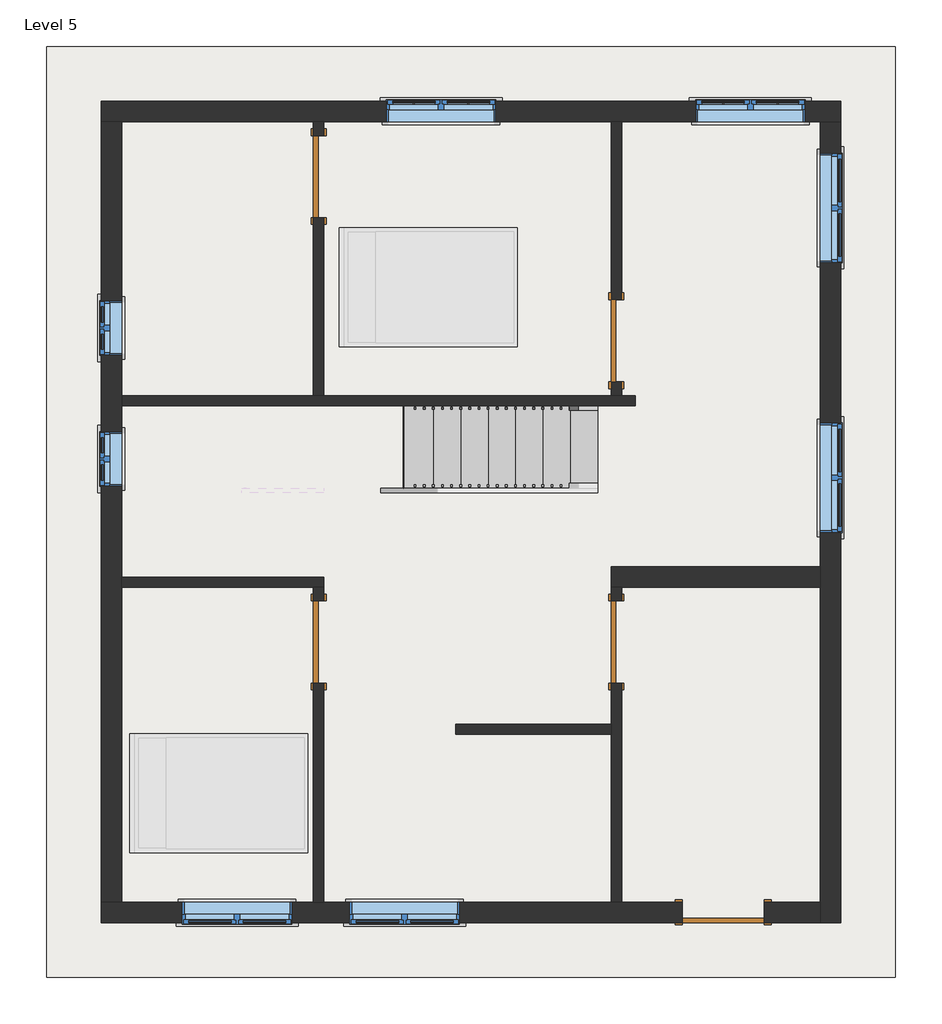
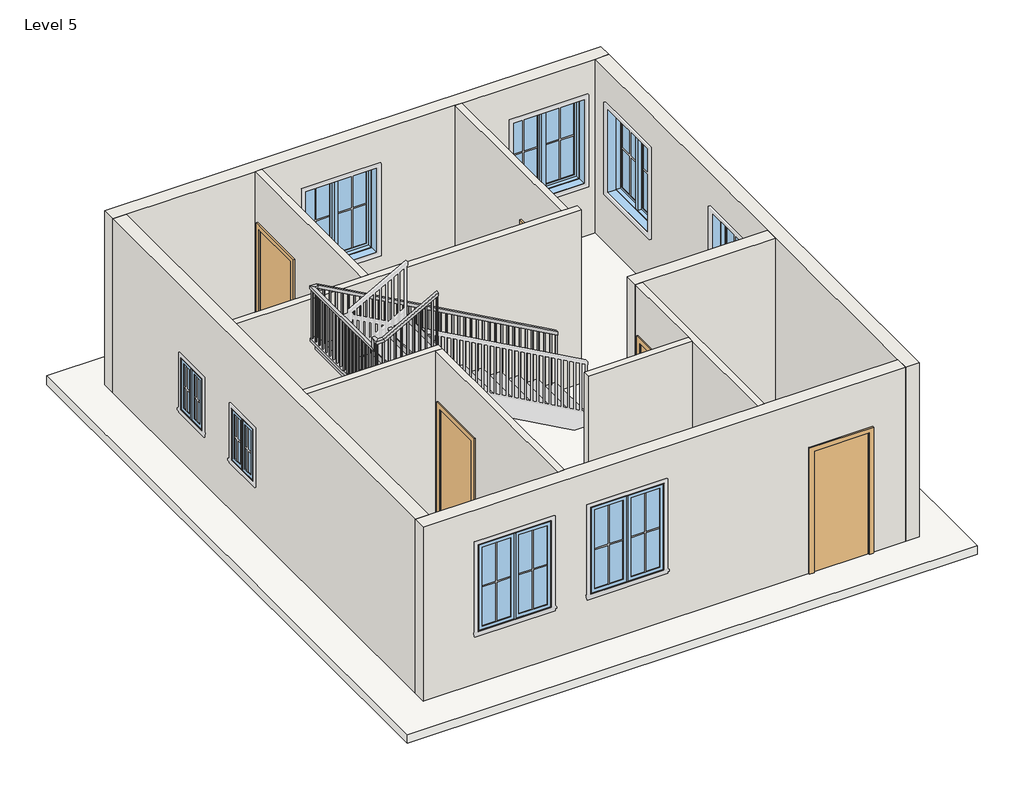
# One storey, part 1 of 2: 12 walls, 8 windows, 5 doors, 1 railing, 1 slab, 1 stair flight.
"""IFC4 building model written with IfcOpenShell, lengths in millimetres."""

from ifc_helpers import new_model, si_unit, frame, origin, place, context, project, spatial, polyline, outline, extrude, faceted_brep, transform, mapped, element, save
from components import door_e5f9f3c4, door_305aa2a5, door_0ca8825f, stair_flight_f65a8a44, window_c417fced, window_8377141f

model = new_model("IFC4")

# Units and contexts
model_context = context("Model", 3, world=origin())
ifc_project = project(units=[si_unit("LENGTHUNIT", "METRE", prefix="MILLI")], contexts=[model_context])

# Site, building, storey
site = spatial("IfcSite", under=ifc_project)
building = spatial("IfcBuilding", under=site)
storey = spatial("IfcBuildingStorey", under=building, Name="Level 5", Elevation=12192.0)

# Doors
placement = place(None, origin())
door_shape = door_e5f9f3c4(model_context)
element("IfcDoor", 1, ObjectType="Single-Flush : 36\" x 84\"", at=placement, inside=storey, context=model_context, shape_type="MappedRepresentation", body=[
    mapped(door_shape, transform((3689.35, 13938.7372886, 12192.0), x_axis=(0.0, 1.0, 0.0), y_axis=(-1.0, 0.0, 0.0), z_axis=(0.0, 0.0, 1.0))),
])
door_2_shape = door_305aa2a5(model_context)
element("IfcDoor", 2, ObjectType="Single-Flush : 36\" x 84\"", at=placement, inside=storey, context=model_context, shape_type="MappedRepresentation", body=[
    mapped(door_2_shape, transform((7004.05, 12109.9372886, 12192.0), x_axis=(0.0, -1.0, 0.0), y_axis=(1.0, 0.0, 0.0), z_axis=(0.0, 0.0, 1.0))),
])
element("IfcDoor", 3, ObjectType="Single-Flush : 36\" x 84\"", at=placement, inside=storey, context=model_context, shape_type="MappedRepresentation", body=[
    mapped(door_2_shape, transform((3689.3519847, 8757.1372886, 12192.0), x_axis=(0.0, -1.0, 0.0), y_axis=(1.0, 0.0, 0.0), z_axis=(0.0, 0.0, 1.0))),
])
element("IfcDoor", 4, ObjectType="Single-Flush : 36\" x 84\"", at=placement, inside=storey, context=model_context, shape_type="MappedRepresentation", body=[
    mapped(door_2_shape, transform((7004.05, 8757.1372886, 12192.0), x_axis=(0.0, -1.0, 0.0), y_axis=(1.0, 0.0, 0.0), z_axis=(0.0, 0.0, 1.0))),
])
door_3_shape = door_0ca8825f(model_context)
element("IfcDoor", 5, ObjectType="Single-Flush : 36\" x 84\"", at=placement, inside=storey, context=model_context, shape_type="MappedRepresentation", body=[
    mapped(door_3_shape, transform((8194.675, 5747.2372886, 12192.0), x_axis=(-1.0, 0.0, 0.0), y_axis=(0.0, -1.0, 0.0), z_axis=(0.0, 0.0, 1.0))),
])

# Railing
element("IfcRailing", 6, ObjectType="Handrail - Rectangular", at=placement, inside=storey, context=model_context, shape_type="SolidModel", body=[
    faceted_brep([(6794.5, 11335.2372886, 13275.7333333), (6794.5, 11335.2372886, 13217.620221), (6794.5, 11386.0372886, 13217.620221), (6794.5, 11386.0372886, 13275.7333333), (2832.1, 11335.2372886, 15477.0666667), (2818.9363978, 11335.2372886, 15426.2666667), (2818.9363978, 11386.0372886, 15426.2666667), (2832.1, 11386.0372886, 15477.0666667), (2768.6, 11335.2372886, 15477.0666667), (2768.6, 11335.2372886, 15426.2666667), (2717.8, 11386.0372886, 15426.2666667), (2717.8, 11386.0372886, 15477.0666667), (2768.6, 9608.0372886, 15477.0666667), (2768.6, 9557.2372886, 15426.2666667), (2717.8, 9557.2372886, 15426.2666667), (2717.8, 9608.0372886, 15477.0666667), (2768.6, 9608.0372886, 15653.4555402), (2768.6, 9557.2372886, 15602.6555402), (2717.8, 9557.2372886, 15602.6555402), (2717.8, 9608.0372886, 15653.4555402), (2768.6, 9531.8372886, 15653.4555402), (2768.6, 9531.8372886, 15602.6555402), (2717.8, 9481.0372886, 15602.6555402), (2717.8, 9481.0372886, 15653.4555402), (2844.8, 9531.8372886, 15653.4555402), (2857.9635773, 9531.8372886, 15602.6555402), (2857.9635773, 9481.0372886, 15602.6555402), (2844.8, 9481.0372886, 15653.4555402), (3746.5019847, 9531.8372886, 16154.4), (3746.5019847, 9481.0372886, 16154.4), (3746.5019847, 9481.0372886, 16096.2869174), (3746.5019847, 9531.8372886, 16096.2869174)], [[[0, 1, 2, 3]], [[1, 0, 4, 5]], [[2, 1, 5, 6]], [[3, 2, 6, 7]], [[0, 3, 7, 4]], [[5, 4, 8, 9]], [[6, 5, 9, 10]], [[7, 6, 10, 11]], [[4, 7, 11, 8]], [[9, 8, 12, 13]], [[10, 9, 13, 14]], [[11, 10, 14, 15]], [[8, 11, 15, 12]], [[13, 12, 16, 17]], [[14, 13, 17, 18]], [[15, 14, 18, 19]], [[12, 15, 19, 16]], [[17, 16, 20, 21]], [[18, 17, 21, 22]], [[19, 18, 22, 23]], [[16, 19, 23, 20]], [[21, 20, 24, 25]], [[22, 21, 25, 26]], [[23, 22, 26, 27]], [[20, 23, 27, 24]], [[28, 29, 30, 31]], [[25, 24, 28, 31]], [[26, 25, 31, 30]], [[27, 26, 30, 29]], [[24, 27, 29, 28]]]),
    extrude(outline(polyline([(16052.1894234, 3667.125), (16041.606113, 3648.075), (15070.6666667, 3648.075), (15070.6666667, 3667.125), (16052.1894234, 3667.125)])), frame((0.0, 9496.9122886, 0.0), z_axis=(0.0, 1.0, 0.0), x_axis=(0.0, 0.0, 1.0)), (0.0, 0.0, 1.0), 19.05),
    extrude(outline(polyline([(15995.7451014, 3565.525), (15985.1617911, 3546.475), (15070.6666667, 3546.475), (15070.6666667, 3565.525), (15995.7451014, 3565.525)])), frame((0.0, 9496.9122886, 0.0), z_axis=(0.0, 1.0, 0.0), x_axis=(0.0, 0.0, 1.0)), (0.0, 0.0, 1.0), 19.05),
    extrude(outline(polyline([(15939.3007795, 3463.925), (15928.7174691, 3444.875), (15070.6666667, 3444.875), (15070.6666667, 3463.925), (15939.3007795, 3463.925)])), frame((0.0, 9496.9122886, 0.0), z_axis=(0.0, 1.0, 0.0), x_axis=(0.0, 0.0, 1.0)), (0.0, 0.0, 1.0), 19.05),
    extrude(outline(polyline([(15882.85609, 3362.325), (15872.2727797, 3343.275), (14901.3333333, 3343.275), (14901.3333333, 3362.325), (15882.85609, 3362.325)])), frame((0.0, 9496.9122886, 0.0), z_axis=(0.0, 1.0, 0.0), x_axis=(0.0, 0.0, 1.0)), (0.0, 0.0, 1.0), 19.05),
    extrude(outline(polyline([(15826.4117681, 3260.725), (15815.8284577, 3241.675), (14901.3333333, 3241.675), (14901.3333333, 3260.725), (15826.4117681, 3260.725)])), frame((0.0, 9496.9122886, 0.0), z_axis=(0.0, 1.0, 0.0), x_axis=(0.0, 0.0, 1.0)), (0.0, 0.0, 1.0), 19.05),
    extrude(outline(polyline([(15769.9674462, 3159.125), (15759.3841358, 3140.075), (14901.3333333, 3140.075), (14901.3333333, 3159.125), (15769.9674462, 3159.125)])), frame((0.0, 9496.9122886, 0.0), z_axis=(0.0, 1.0, 0.0), x_axis=(0.0, 0.0, 1.0)), (0.0, 0.0, 1.0), 19.05),
    extrude(outline(polyline([(15713.5227567, 3057.525), (15702.9394463, 3038.475), (14732.0, 3038.475), (14732.0, 3057.525), (15713.5227567, 3057.525)])), frame((0.0, 9496.9122886, 0.0), z_axis=(0.0, 1.0, 0.0), x_axis=(0.0, 0.0, 1.0)), (0.0, 0.0, 1.0), 19.05),
    extrude(outline(polyline([(15657.0784348, 2955.925), (15646.4951244, 2936.875), (14732.0, 2936.875), (14732.0, 2955.925), (15657.0784348, 2955.925)])), frame((0.0, 9496.9122886, 0.0), z_axis=(0.0, 1.0, 0.0), x_axis=(0.0, 0.0, 1.0)), (0.0, 0.0, 1.0), 19.05),
    extrude(outline(polyline([(15600.6341128, 2854.325), (15590.0508025, 2835.275), (14732.0, 2835.275), (14732.0, 2854.325), (15600.6341128, 2854.325)])), frame((0.0, 9496.9122886, 0.0), z_axis=(0.0, 1.0, 0.0), x_axis=(0.0, 0.0, 1.0)), (0.0, 0.0, 1.0), 19.05),
    extrude(outline(polyline([(2733.675, 9541.3622886), (2752.725, 9541.3622886), (2752.725, 9522.3122886), (2733.675, 9522.3122886), (2733.675, 9541.3622886)])), frame((0.0, 0.0, 14562.6666667), z_axis=(0.0, 0.0, 1.0), x_axis=(1.0, 0.0, 0.0)), (0.0, 0.0, 1.0), 1039.9888736),
    extrude(outline(polyline([(2733.675, 9642.9622886), (2752.725, 9642.9622886), (2752.725, 9623.9122886), (2733.675, 9623.9122886), (2733.675, 9642.9622886)])), frame((0.0, 0.0, 14562.6666667), z_axis=(0.0, 0.0, 1.0), x_axis=(1.0, 0.0, 0.0)), (0.0, 0.0, 1.0), 863.6),
    extrude(outline(polyline([(2733.675, 9744.5622886), (2752.725, 9744.5622886), (2752.725, 9725.5122886), (2733.675, 9725.5122886), (2733.675, 9744.5622886)])), frame((0.0, 0.0, 14562.6666667), z_axis=(0.0, 0.0, 1.0), x_axis=(1.0, 0.0, 0.0)), (0.0, 0.0, 1.0), 863.6),
    extrude(outline(polyline([(2733.675, 9846.1622886), (2752.725, 9846.1622886), (2752.725, 9827.1122886), (2733.675, 9827.1122886), (2733.675, 9846.1622886)])), frame((0.0, 0.0, 14562.6666667), z_axis=(0.0, 0.0, 1.0), x_axis=(1.0, 0.0, 0.0)), (0.0, 0.0, 1.0), 863.6),
    extrude(outline(polyline([(2733.675, 9947.7622886), (2752.725, 9947.7622886), (2752.725, 9928.7122886), (2733.675, 9928.7122886), (2733.675, 9947.7622886)])), frame((0.0, 0.0, 14562.6666667), z_axis=(0.0, 0.0, 1.0), x_axis=(1.0, 0.0, 0.0)), (0.0, 0.0, 1.0), 863.6),
    extrude(outline(polyline([(2733.675, 10049.3622886), (2752.725, 10049.3622886), (2752.725, 10030.3122886), (2733.675, 10030.3122886), (2733.675, 10049.3622886)])), frame((0.0, 0.0, 14562.6666667), z_axis=(0.0, 0.0, 1.0), x_axis=(1.0, 0.0, 0.0)), (0.0, 0.0, 1.0), 863.6),
    extrude(outline(polyline([(2733.675, 10150.9622886), (2752.725, 10150.9622886), (2752.725, 10131.9122886), (2733.675, 10131.9122886), (2733.675, 10150.9622886)])), frame((0.0, 0.0, 14562.6666667), z_axis=(0.0, 0.0, 1.0), x_axis=(1.0, 0.0, 0.0)), (0.0, 0.0, 1.0), 863.6),
    extrude(outline(polyline([(2733.675, 10252.5622886), (2752.725, 10252.5622886), (2752.725, 10233.5122886), (2733.675, 10233.5122886), (2733.675, 10252.5622886)])), frame((0.0, 0.0, 14562.6666667), z_axis=(0.0, 0.0, 1.0), x_axis=(1.0, 0.0, 0.0)), (0.0, 0.0, 1.0), 863.6),
    extrude(outline(polyline([(2733.675, 10354.1622886), (2752.725, 10354.1622886), (2752.725, 10335.1122886), (2733.675, 10335.1122886), (2733.675, 10354.1622886)])), frame((0.0, 0.0, 14562.6666667), z_axis=(0.0, 0.0, 1.0), x_axis=(1.0, 0.0, 0.0)), (0.0, 0.0, 1.0), 863.6),
    extrude(outline(polyline([(2733.675, 10455.7622886), (2752.725, 10455.7622886), (2752.725, 10436.7122886), (2733.675, 10436.7122886), (2733.675, 10455.7622886)])), frame((0.0, 0.0, 14562.6666667), z_axis=(0.0, 0.0, 1.0), x_axis=(1.0, 0.0, 0.0)), (0.0, 0.0, 1.0), 863.6),
    extrude(outline(polyline([(2733.675, 10557.3622886), (2752.725, 10557.3622886), (2752.725, 10538.3122886), (2733.675, 10538.3122886), (2733.675, 10557.3622886)])), frame((0.0, 0.0, 14562.6666667), z_axis=(0.0, 0.0, 1.0), x_axis=(1.0, 0.0, 0.0)), (0.0, 0.0, 1.0), 863.6),
    extrude(outline(polyline([(2733.675, 10658.9622886), (2752.725, 10658.9622886), (2752.725, 10639.9122886), (2733.675, 10639.9122886), (2733.675, 10658.9622886)])), frame((0.0, 0.0, 14562.6666667), z_axis=(0.0, 0.0, 1.0), x_axis=(1.0, 0.0, 0.0)), (0.0, 0.0, 1.0), 863.6),
    extrude(outline(polyline([(2733.675, 10760.5622886), (2752.725, 10760.5622886), (2752.725, 10741.5122886), (2733.675, 10741.5122886), (2733.675, 10760.5622886)])), frame((0.0, 0.0, 14562.6666667), z_axis=(0.0, 0.0, 1.0), x_axis=(1.0, 0.0, 0.0)), (0.0, 0.0, 1.0), 863.6),
    extrude(outline(polyline([(2733.675, 10862.1622886), (2752.725, 10862.1622886), (2752.725, 10843.1122886), (2733.675, 10843.1122886), (2733.675, 10862.1622886)])), frame((0.0, 0.0, 14562.6666667), z_axis=(0.0, 0.0, 1.0), x_axis=(1.0, 0.0, 0.0)), (0.0, 0.0, 1.0), 863.6),
    extrude(outline(polyline([(2733.675, 10963.7622886), (2752.725, 10963.7622886), (2752.725, 10944.7122886), (2733.675, 10944.7122886), (2733.675, 10963.7622886)])), frame((0.0, 0.0, 14562.6666667), z_axis=(0.0, 0.0, 1.0), x_axis=(1.0, 0.0, 0.0)), (0.0, 0.0, 1.0), 863.6),
    extrude(outline(polyline([(2733.675, 11065.3622886), (2752.725, 11065.3622886), (2752.725, 11046.3122886), (2733.675, 11046.3122886), (2733.675, 11065.3622886)])), frame((0.0, 0.0, 14562.6666667), z_axis=(0.0, 0.0, 1.0), x_axis=(1.0, 0.0, 0.0)), (0.0, 0.0, 1.0), 863.6),
    extrude(outline(polyline([(2733.675, 11166.9622886), (2752.725, 11166.9622886), (2752.725, 11147.9122886), (2733.675, 11147.9122886), (2733.675, 11166.9622886)])), frame((0.0, 0.0, 14562.6666667), z_axis=(0.0, 0.0, 1.0), x_axis=(1.0, 0.0, 0.0)), (0.0, 0.0, 1.0), 863.6),
    extrude(outline(polyline([(2733.675, 11268.5622886), (2752.725, 11268.5622886), (2752.725, 11249.5122886), (2733.675, 11249.5122886), (2733.675, 11268.5622886)])), frame((0.0, 0.0, 14562.6666667), z_axis=(0.0, 0.0, 1.0), x_axis=(1.0, 0.0, 0.0)), (0.0, 0.0, 1.0), 863.6),
    extrude(outline(polyline([(15413.6618876, 2841.625), (15424.245221, 2822.575), (14562.6666667, 2822.575), (14562.6666667, 2841.625), (15413.6618876, 2841.625)])), frame((0.0, 11351.1122886, 0.0), z_axis=(0.0, 1.0, 0.0), x_axis=(0.0, 0.0, 1.0)), (0.0, 0.0, 1.0), 19.05),
    extrude(outline(polyline([(15357.2174432, 2943.225), (15367.8007765, 2924.175), (14393.3333333, 2924.175), (14393.3333333, 2943.225), (15357.2174432, 2943.225)])), frame((0.0, 11351.1122886, 0.0), z_axis=(0.0, 1.0, 0.0), x_axis=(0.0, 0.0, 1.0)), (0.0, 0.0, 1.0), 19.05),
    extrude(outline(polyline([(15300.7729988, 3044.825), (15311.3563321, 3025.775), (14393.3333333, 3025.775), (14393.3333333, 3044.825), (15300.7729988, 3044.825)])), frame((0.0, 11351.1122886, 0.0), z_axis=(0.0, 1.0, 0.0), x_axis=(0.0, 0.0, 1.0)), (0.0, 0.0, 1.0), 19.05),
    extrude(outline(polyline([(15244.3285543, 3146.425), (15254.9118876, 3127.375), (14393.3333333, 3127.375), (14393.3333333, 3146.425), (15244.3285543, 3146.425)])), frame((0.0, 11351.1122886, 0.0), z_axis=(0.0, 1.0, 0.0), x_axis=(0.0, 0.0, 1.0)), (0.0, 0.0, 1.0), 19.05),
    extrude(outline(polyline([(15187.8841099, 3248.025), (15198.4674432, 3228.975), (14224.0, 3228.975), (14224.0, 3248.025), (15187.8841099, 3248.025)])), frame((0.0, 11351.1122886, 0.0), z_axis=(0.0, 1.0, 0.0), x_axis=(0.0, 0.0, 1.0)), (0.0, 0.0, 1.0), 19.05),
    extrude(outline(polyline([(15131.4396654, 3349.625), (15142.0229988, 3330.575), (14224.0, 3330.575), (14224.0, 3349.625), (15131.4396654, 3349.625)])), frame((0.0, 11351.1122886, 0.0), z_axis=(0.0, 1.0, 0.0), x_axis=(0.0, 0.0, 1.0)), (0.0, 0.0, 1.0), 19.05),
    extrude(outline(polyline([(15074.995221, 3451.225), (15085.5785543, 3432.175), (14224.0, 3432.175), (14224.0, 3451.225), (15074.995221, 3451.225)])), frame((0.0, 11351.1122886, 0.0), z_axis=(0.0, 1.0, 0.0), x_axis=(0.0, 0.0, 1.0)), (0.0, 0.0, 1.0), 19.05),
    extrude(outline(polyline([(15018.5507765, 3552.825), (15029.1341099, 3533.775), (14054.6666667, 3533.775), (14054.6666667, 3552.825), (15018.5507765, 3552.825)])), frame((0.0, 11351.1122886, 0.0), z_axis=(0.0, 1.0, 0.0), x_axis=(0.0, 0.0, 1.0)), (0.0, 0.0, 1.0), 19.05),
    extrude(outline(polyline([(14962.1063321, 3654.425), (14972.6896654, 3635.375), (14054.6666667, 3635.375), (14054.6666667, 3654.425), (14962.1063321, 3654.425)])), frame((0.0, 11351.1122886, 0.0), z_axis=(0.0, 1.0, 0.0), x_axis=(0.0, 0.0, 1.0)), (0.0, 0.0, 1.0), 19.05),
    extrude(outline(polyline([(14905.6618876, 3756.025), (14916.245221, 3736.975), (14054.6666667, 3736.975), (14054.6666667, 3756.025), (14905.6618876, 3756.025)])), frame((0.0, 11351.1122886, 0.0), z_axis=(0.0, 1.0, 0.0), x_axis=(0.0, 0.0, 1.0)), (0.0, 0.0, 1.0), 19.05),
    extrude(outline(polyline([(14849.2174432, 3857.625), (14859.8007765, 3838.575), (13885.3333333, 3838.575), (13885.3333333, 3857.625), (14849.2174432, 3857.625)])), frame((0.0, 11351.1122886, 0.0), z_axis=(0.0, 1.0, 0.0), x_axis=(0.0, 0.0, 1.0)), (0.0, 0.0, 1.0), 19.05),
    extrude(outline(polyline([(14792.7729988, 3959.225), (14803.3563321, 3940.175), (13885.3333333, 3940.175), (13885.3333333, 3959.225), (14792.7729988, 3959.225)])), frame((0.0, 11351.1122886, 0.0), z_axis=(0.0, 1.0, 0.0), x_axis=(0.0, 0.0, 1.0)), (0.0, 0.0, 1.0), 19.05),
    extrude(outline(polyline([(14736.3285543, 4060.825), (14746.9118876, 4041.775), (13885.3333333, 4041.775), (13885.3333333, 4060.825), (14736.3285543, 4060.825)])), frame((0.0, 11351.1122886, 0.0), z_axis=(0.0, 1.0, 0.0), x_axis=(0.0, 0.0, 1.0)), (0.0, 0.0, 1.0), 19.05),
    extrude(outline(polyline([(14679.8841099, 4162.425), (14690.4674432, 4143.375), (13716.0, 4143.375), (13716.0, 4162.425), (14679.8841099, 4162.425)])), frame((0.0, 11351.1122886, 0.0), z_axis=(0.0, 1.0, 0.0), x_axis=(0.0, 0.0, 1.0)), (0.0, 0.0, 1.0), 19.05),
    extrude(outline(polyline([(14623.4396654, 4264.025), (14634.0229988, 4244.975), (13716.0, 4244.975), (13716.0, 4264.025), (14623.4396654, 4264.025)])), frame((0.0, 11351.1122886, 0.0), z_axis=(0.0, 1.0, 0.0), x_axis=(0.0, 0.0, 1.0)), (0.0, 0.0, 1.0), 19.05),
    extrude(outline(polyline([(14566.995221, 4365.625), (14577.5785543, 4346.575), (13716.0, 4346.575), (13716.0, 4365.625), (14566.995221, 4365.625)])), frame((0.0, 11351.1122886, 0.0), z_axis=(0.0, 1.0, 0.0), x_axis=(0.0, 0.0, 1.0)), (0.0, 0.0, 1.0), 19.05),
    extrude(outline(polyline([(14510.5507765, 4467.225), (14521.1341099, 4448.175), (13546.6666667, 4448.175), (13546.6666667, 4467.225), (14510.5507765, 4467.225)])), frame((0.0, 11351.1122886, 0.0), z_axis=(0.0, 1.0, 0.0), x_axis=(0.0, 0.0, 1.0)), (0.0, 0.0, 1.0), 19.05),
    extrude(outline(polyline([(14454.1063321, 4568.825), (14464.6896654, 4549.775), (13546.6666667, 4549.775), (13546.6666667, 4568.825), (14454.1063321, 4568.825)])), frame((0.0, 11351.1122886, 0.0), z_axis=(0.0, 1.0, 0.0), x_axis=(0.0, 0.0, 1.0)), (0.0, 0.0, 1.0), 19.05),
    extrude(outline(polyline([(14397.6618876, 4670.425), (14408.245221, 4651.375), (13546.6666667, 4651.375), (13546.6666667, 4670.425), (14397.6618876, 4670.425)])), frame((0.0, 11351.1122886, 0.0), z_axis=(0.0, 1.0, 0.0), x_axis=(0.0, 0.0, 1.0)), (0.0, 0.0, 1.0), 19.05),
    extrude(outline(polyline([(14341.2174432, 4772.025), (14351.8007765, 4752.975), (13377.3333333, 4752.975), (13377.3333333, 4772.025), (14341.2174432, 4772.025)])), frame((0.0, 11351.1122886, 0.0), z_axis=(0.0, 1.0, 0.0), x_axis=(0.0, 0.0, 1.0)), (0.0, 0.0, 1.0), 19.05),
    extrude(outline(polyline([(14284.7729988, 4873.625), (14295.3563321, 4854.575), (13377.3333333, 4854.575), (13377.3333333, 4873.625), (14284.7729988, 4873.625)])), frame((0.0, 11351.1122886, 0.0), z_axis=(0.0, 1.0, 0.0), x_axis=(0.0, 0.0, 1.0)), (0.0, 0.0, 1.0), 19.05),
    extrude(outline(polyline([(14228.3285543, 4975.225), (14238.9118876, 4956.175), (13377.3333333, 4956.175), (13377.3333333, 4975.225), (14228.3285543, 4975.225)])), frame((0.0, 11351.1122886, 0.0), z_axis=(0.0, 1.0, 0.0), x_axis=(0.0, 0.0, 1.0)), (0.0, 0.0, 1.0), 19.05),
    extrude(outline(polyline([(14171.8841099, 5076.825), (14182.4674432, 5057.775), (13208.0, 5057.775), (13208.0, 5076.825), (14171.8841099, 5076.825)])), frame((0.0, 11351.1122886, 0.0), z_axis=(0.0, 1.0, 0.0), x_axis=(0.0, 0.0, 1.0)), (0.0, 0.0, 1.0), 19.05),
    extrude(outline(polyline([(14115.4396654, 5178.425), (14126.0229988, 5159.375), (13208.0, 5159.375), (13208.0, 5178.425), (14115.4396654, 5178.425)])), frame((0.0, 11351.1122886, 0.0), z_axis=(0.0, 1.0, 0.0), x_axis=(0.0, 0.0, 1.0)), (0.0, 0.0, 1.0), 19.05),
    extrude(outline(polyline([(14058.995221, 5280.025), (14069.5785543, 5260.975), (13208.0, 5260.975), (13208.0, 5280.025), (14058.995221, 5280.025)])), frame((0.0, 11351.1122886, 0.0), z_axis=(0.0, 1.0, 0.0), x_axis=(0.0, 0.0, 1.0)), (0.0, 0.0, 1.0), 19.05),
    extrude(outline(polyline([(14002.5507765, 5381.625), (14013.1341099, 5362.575), (13038.6666667, 5362.575), (13038.6666667, 5381.625), (14002.5507765, 5381.625)])), frame((0.0, 11351.1122886, 0.0), z_axis=(0.0, 1.0, 0.0), x_axis=(0.0, 0.0, 1.0)), (0.0, 0.0, 1.0), 19.05),
    extrude(outline(polyline([(13946.1063321, 5483.225), (13956.6896654, 5464.175), (13038.6666667, 5464.175), (13038.6666667, 5483.225), (13946.1063321, 5483.225)])), frame((0.0, 11351.1122886, 0.0), z_axis=(0.0, 1.0, 0.0), x_axis=(0.0, 0.0, 1.0)), (0.0, 0.0, 1.0), 19.05),
    extrude(outline(polyline([(13889.6618876, 5584.825), (13900.245221, 5565.775), (13038.6666667, 5565.775), (13038.6666667, 5584.825), (13889.6618876, 5584.825)])), frame((0.0, 11351.1122886, 0.0), z_axis=(0.0, 1.0, 0.0), x_axis=(0.0, 0.0, 1.0)), (0.0, 0.0, 1.0), 19.05),
    extrude(outline(polyline([(13833.2174432, 5686.425), (13843.8007765, 5667.375), (12869.3333333, 5667.375), (12869.3333333, 5686.425), (13833.2174432, 5686.425)])), frame((0.0, 11351.1122886, 0.0), z_axis=(0.0, 1.0, 0.0), x_axis=(0.0, 0.0, 1.0)), (0.0, 0.0, 1.0), 19.05),
    extrude(outline(polyline([(13776.7729988, 5788.025), (13787.3563321, 5768.975), (12869.3333333, 5768.975), (12869.3333333, 5788.025), (13776.7729988, 5788.025)])), frame((0.0, 11351.1122886, 0.0), z_axis=(0.0, 1.0, 0.0), x_axis=(0.0, 0.0, 1.0)), (0.0, 0.0, 1.0), 19.05),
    extrude(outline(polyline([(13720.3285543, 5889.625), (13730.9118876, 5870.575), (12869.3333333, 5870.575), (12869.3333333, 5889.625), (13720.3285543, 5889.625)])), frame((0.0, 11351.1122886, 0.0), z_axis=(0.0, 1.0, 0.0), x_axis=(0.0, 0.0, 1.0)), (0.0, 0.0, 1.0), 19.05),
    extrude(outline(polyline([(13663.8841099, 5991.225), (13674.4674432, 5972.175), (12700.0, 5972.175), (12700.0, 5991.225), (13663.8841099, 5991.225)])), frame((0.0, 11351.1122886, 0.0), z_axis=(0.0, 1.0, 0.0), x_axis=(0.0, 0.0, 1.0)), (0.0, 0.0, 1.0), 19.05),
    extrude(outline(polyline([(13607.4396654, 6092.825), (13618.0229988, 6073.775), (12700.0, 6073.775), (12700.0, 6092.825), (13607.4396654, 6092.825)])), frame((0.0, 11351.1122886, 0.0), z_axis=(0.0, 1.0, 0.0), x_axis=(0.0, 0.0, 1.0)), (0.0, 0.0, 1.0), 19.05),
    extrude(outline(polyline([(13550.995221, 6194.425), (13561.5785543, 6175.375), (12700.0, 6175.375), (12700.0, 6194.425), (13550.995221, 6194.425)])), frame((0.0, 11351.1122886, 0.0), z_axis=(0.0, 1.0, 0.0), x_axis=(0.0, 0.0, 1.0)), (0.0, 0.0, 1.0), 19.05),
    extrude(outline(polyline([(13494.5507765, 6296.025), (13505.1341099, 6276.975), (12530.6666667, 6276.975), (12530.6666667, 6296.025), (13494.5507765, 6296.025)])), frame((0.0, 11351.1122886, 0.0), z_axis=(0.0, 1.0, 0.0), x_axis=(0.0, 0.0, 1.0)), (0.0, 0.0, 1.0), 19.05),
    extrude(outline(polyline([(13438.1063321, 6397.625), (13448.6896654, 6378.575), (12530.6666667, 6378.575), (12530.6666667, 6397.625), (13438.1063321, 6397.625)])), frame((0.0, 11351.1122886, 0.0), z_axis=(0.0, 1.0, 0.0), x_axis=(0.0, 0.0, 1.0)), (0.0, 0.0, 1.0), 19.05),
    extrude(outline(polyline([(13381.6618876, 6499.225), (13392.245221, 6480.175), (12530.6666667, 6480.175), (12530.6666667, 6499.225), (13381.6618876, 6499.225)])), frame((0.0, 11351.1122886, 0.0), z_axis=(0.0, 1.0, 0.0), x_axis=(0.0, 0.0, 1.0)), (0.0, 0.0, 1.0), 19.05),
    extrude(outline(polyline([(13325.2174432, 6600.825), (13335.8007765, 6581.775), (12361.3333333, 6581.775), (12361.3333333, 6600.825), (13325.2174432, 6600.825)])), frame((0.0, 11351.1122886, 0.0), z_axis=(0.0, 1.0, 0.0), x_axis=(0.0, 0.0, 1.0)), (0.0, 0.0, 1.0), 19.05),
    extrude(outline(polyline([(13268.7729988, 6702.425), (13279.3563321, 6683.375), (12361.3333333, 6683.375), (12361.3333333, 6702.425), (13268.7729988, 6702.425)])), frame((0.0, 11351.1122886, 0.0), z_axis=(0.0, 1.0, 0.0), x_axis=(0.0, 0.0, 1.0)), (0.0, 0.0, 1.0), 19.05),
    extrude(outline(polyline([(2733.675, 9515.9622886), (2752.725, 9515.9622886), (2752.725, 9496.9122886), (2733.675, 9496.9122886), (2733.675, 9515.9622886)])), frame((0.0, 0.0, 14562.6666667), z_axis=(0.0, 0.0, 1.0), x_axis=(1.0, 0.0, 0.0)), (0.0, 0.0, 1.0), 1039.9888736),
    extrude(outline(polyline([(2752.725, 11370.1622886), (2752.725, 11351.1122886), (2733.675, 11351.1122886), (2733.675, 11370.1622886), (2752.725, 11370.1622886)])), frame((0.0, 0.0, 14562.6666667), z_axis=(0.0, 0.0, 1.0), x_axis=(1.0, 0.0, 0.0)), (0.0, 0.0, 1.0), 863.6),
    extrude(outline(polyline([(16096.2869174, 3746.5019847), (16085.703607, 3727.4519847), (15070.6666667, 3727.4519847), (15070.6666667, 3746.5019847), (16096.2869174, 3746.5019847)])), frame((0.0, 9496.9122886, 0.0), z_axis=(0.0, 1.0, 0.0), x_axis=(0.0, 0.0, 1.0)), (0.0, 0.0, 1.0), 19.05),
    extrude(outline(polyline([(13217.620221, 6794.5), (13228.2035543, 6775.45), (12361.3333333, 6775.45), (12361.3333333, 6794.5), (13217.620221, 6794.5)])), frame((0.0, 11351.1122886, 0.0), z_axis=(0.0, 1.0, 0.0), x_axis=(0.0, 0.0, 1.0)), (0.0, 0.0, 1.0), 19.05),
])

# Slab
element("IfcSlab", 7, ObjectType="Generic - 12\"", at=placement, inside=storey, context=model_context, shape_type="SweptSolid", body=[
    extrude(outline(polyline([(10109.2, 15386.5372886), (10109.2, 5023.3372886), (660.4, 5023.3372886), (660.4, 15386.5372886), (10109.2, 15386.5372886)])), frame((0.0, 0.0, 12039.6), z_axis=(0.0, 0.0, 1.0), x_axis=(1.0, 0.0, 0.0)), (0.0, 0.0, 1.0), 152.4),
])

# Stair flight
stair_flight_shape = stair_flight_f65a8a44(model_context)
element("IfcStairFlight", 8, ObjectType="2\" Tread 1\" Nosing 1/4\" Riser", at=placement, inside=storey, context=model_context, shape_type="MappedRepresentation", body=[
    mapped(stair_flight_shape, transform((0.0, 0.0, 0.0), x_axis=(1.0, 0.0, 0.0), y_axis=(0.0, 1.0, 0.0), z_axis=(0.0, 0.0, 1.0))),
])

# Walls
element("IfcWall", 9, ObjectType="Generic - 5\"", at=placement, inside=storey, context=model_context, shape_type="SweptSolid", body=[
    extrude(outline(polyline([(14548.3372886, 12192.0), (14395.9372886, 12192.0), (14395.9372886, 14325.6), (13481.5372886, 14325.6), (13481.5372886, 12192.0), (11500.3372886, 12192.0), (11500.3372886, 15240.0), (14548.3372886, 15240.0), (14548.3372886, 12192.0)])), frame((3632.2, 0.0, 0.0), z_axis=(1.0, 0.0, 0.0), x_axis=(0.0, 1.0, 0.0)), (0.0, 0.0, 1.0), 114.3),
])
element("IfcWall", 10, ObjectType="Generic - 5\"", at=placement, inside=storey, context=model_context, shape_type="SweptSolid", body=[
    extrude(outline(polyline([(11652.7372886, 14325.6), (11652.7372886, 12192.0), (11500.3372886, 12192.0), (11500.3372886, 15240.0), (14548.3372886, 15240.0), (14548.3372886, 12192.0), (12567.1372886, 12192.0), (12567.1372886, 14325.6), (11652.7372886, 14325.6)])), frame((6946.9, 0.0, 0.0), z_axis=(1.0, 0.0, 0.0), x_axis=(0.0, 1.0, 0.0)), (0.0, 0.0, 1.0), 114.3),
])
element("IfcWall", 11, ObjectType="Generic - 5\"", at=placement, inside=storey, context=model_context, shape_type="Brep", body=[
    faceted_brep([(1498.6, 11386.0372886, 12192.0), (7213.6, 11386.0372886, 12192.0), (7213.6, 11386.0372886, 15240.0), (1498.6, 11386.0372886, 15240.0), (1498.6, 11500.3372886, 12192.0), (1498.6, 11500.3372886, 15240.0), (3632.2, 11500.3372886, 15240.0), (3746.5, 11500.3372886, 15240.0), (6946.9, 11500.3372886, 15240.0), (7061.2, 11500.3372886, 15240.0), (7213.6, 11500.3372886, 15240.0), (7213.6, 11500.3372886, 12192.0), (7061.2, 11500.3372886, 12192.0), (6946.9, 11500.3372886, 12192.0), (3746.5, 11500.3372886, 12192.0), (3632.2, 11500.3372886, 12192.0)], [[[0, 1, 2, 3]], [[4, 5, 6, 7, 8, 9, 10, 11, 12, 13, 14, 15]], [[1, 0, 4, 15, 14, 13, 12, 11]], [[2, 1, 11, 10]], [[3, 2, 10, 9, 8, 7, 6, 5]], [[0, 3, 5, 4]]]),
])
element("IfcWall", 12, ObjectType="Generic - 5\"", at=placement, inside=storey, context=model_context, shape_type="Brep", body=[
    faceted_brep([(1498.6, 9366.7372886, 12192.0), (3632.2019847, 9366.7372886, 12192.0), (3746.5019847, 9366.7372886, 12192.0), (3746.5019847, 9366.7372886, 15240.0), (3632.2019847, 9366.7372886, 15240.0), (1498.6, 9366.7372886, 15240.0), (1498.6, 9481.0372886, 12192.0), (1498.6, 9481.0372886, 15240.0), (3746.5019847, 9481.0372886, 15240.0), (3746.5019847, 9481.0372886, 12192.0)], [[[0, 1, 2, 3, 4, 5]], [[6, 7, 8, 9]], [[2, 1, 0, 6, 9]], [[5, 4, 3, 8, 7]], [[0, 5, 7, 6]], [[3, 2, 9, 8]]]),
])
element("IfcWall", 13, ObjectType="Generic - 5\"", at=placement, inside=storey, context=model_context, shape_type="SweptSolid", body=[
    extrude(outline(polyline([(8299.9372886, 14325.6), (8299.9372886, 12192.0), (5861.5372886, 12192.0), (5861.5372886, 15240.0), (9366.7372886, 15240.0), (9366.7372886, 12192.0), (9214.3372886, 12192.0), (9214.3372886, 14325.6), (8299.9372886, 14325.6)])), frame((3632.2019847, 0.0, 0.0), z_axis=(1.0, 0.0, 0.0), x_axis=(0.0, 1.0, 0.0)), (0.0, 0.0, 1.0), 114.3),
])
element("IfcWall", 14, ObjectType="Generic - 5\"", at=placement, inside=storey, context=model_context, shape_type="Brep", body=[
    faceted_brep([(7061.2, 5861.5372886, 12192.0), (7061.2, 8299.9372886, 12192.0), (7061.2, 8299.9372886, 14325.6), (7061.2, 9214.3372886, 14325.6), (7061.2, 9214.3372886, 12192.0), (7061.2, 9366.7372886, 12192.0), (7061.2, 9366.7372886, 15240.0), (7061.2, 5861.5372886, 15240.0), (6946.9, 8299.9372886, 14325.6), (6946.9, 8299.9372886, 12192.0), (6946.9, 7842.7372886, 12192.0), (6946.9, 7728.4372886, 12192.0), (6946.9, 5861.5372886, 12192.0), (6946.9, 5861.5372886, 15240.0), (6946.9, 7728.4372886, 15240.0), (6946.9, 7842.7372886, 15240.0), (6946.9, 9366.7372886, 15240.0), (6946.9, 9366.7372886, 12192.0), (6946.9, 9214.3372886, 12192.0), (6946.9, 9214.3372886, 14325.6)], [[[0, 1, 2, 3, 4, 5, 6, 7]], [[8, 9, 10, 11, 12, 13, 14, 15, 16, 17, 18, 19]], [[18, 17, 5, 4]], [[12, 11, 10, 9, 1, 0]], [[7, 6, 16, 15, 14, 13]], [[0, 7, 13, 12]], [[6, 5, 17, 16]], [[2, 1, 9, 8]], [[3, 2, 8, 19]], [[4, 3, 19, 18]]]),
])
element("IfcWall", 15, ObjectType="Generic - 5\"", at=placement, inside=storey, context=model_context, shape_type="SweptSolid", body=[
    extrude(outline(polyline([(5215.2207778, 7842.7372886), (6946.9, 7842.7372886), (6946.9, 7728.4372886), (5215.2207778, 7728.4372886), (5215.2207778, 7842.7372886)])), frame((0.0, 0.0, 12192.0), z_axis=(0.0, 0.0, 1.0), x_axis=(1.0, 0.0, 0.0)), (0.0, 0.0, 1.0), 3048.0),
])
element("IfcWall", 16, ObjectType="Generic - 8\"", at=placement, inside=storey, context=model_context, shape_type="Brep", body=[
    faceted_brep([(1270.0, 14548.3372886, 12192.0), (1498.6, 14548.3372886, 12192.0), (3632.2, 14548.3372886, 12192.0), (3746.5, 14548.3372886, 12192.0), (6946.9, 14548.3372886, 12192.0), (7061.2, 14548.3372886, 12192.0), (9271.0, 14548.3372886, 12192.0), (9499.6, 14548.3372886, 12192.0), (9499.6, 14548.3372886, 15240.0), (9271.0, 14548.3372886, 15240.0), (7061.2, 14548.3372886, 15240.0), (6946.9, 14548.3372886, 15240.0), (3746.5, 14548.3372886, 15240.0), (3632.2, 14548.3372886, 15240.0), (1498.6, 14548.3372886, 15240.0), (1270.0, 14548.3372886, 15240.0), (9105.9, 14548.3372886, 14630.4), (9105.9, 14548.3372886, 13106.4), (7886.7, 14548.3372886, 13106.4), (7886.7, 14548.3372886, 14630.4), (5662.6125, 14548.3372886, 14630.4), (5662.6125, 14548.3372886, 13106.4), (4443.4125, 14548.3372886, 13106.4), (4443.4125, 14548.3372886, 14630.4), (1270.0, 14776.9372886, 12192.0), (1270.0, 14776.9372886, 15240.0), (9499.6, 14776.9372886, 15240.0), (9499.6, 14776.9372886, 12192.0), (9105.9, 14776.9372886, 14630.4), (7886.7, 14776.9372886, 14630.4), (7886.7, 14776.9372886, 13106.4), (9105.9, 14776.9372886, 13106.4), (5662.6125, 14776.9372886, 14630.4), (4443.4125, 14776.9372886, 14630.4), (4443.4125, 14776.9372886, 13106.4), (5662.6125, 14776.9372886, 13106.4)], [[[0, 1, 2, 3, 4, 5, 6, 7, 8, 9, 10, 11, 12, 13, 14, 15], [16, 17, 18, 19], [20, 21, 22, 23]], [[24, 25, 26, 27], [28, 29, 30, 31], [32, 33, 34, 35]], [[7, 6, 5, 4, 3, 2, 1, 0, 24, 27]], [[8, 7, 27, 26]], [[0, 15, 25, 24]], [[17, 16, 28, 31]], [[18, 17, 31, 30]], [[19, 18, 30, 29]], [[16, 19, 29, 28]], [[21, 20, 32, 35]], [[22, 21, 35, 34]], [[23, 22, 34, 33]], [[20, 23, 33, 32]], [[15, 14, 13, 12, 11, 10, 9, 8, 26, 25]]]),
])
element("IfcWall", 17, ObjectType="Generic - 8\"", at=placement, inside=storey, context=model_context, shape_type="Brep", body=[
    faceted_brep([(9271.0, 14548.3372886, 12192.0), (9271.0, 9595.3372886, 12192.0), (9271.0, 9366.7372886, 12192.0), (9271.0, 5861.5372886, 12192.0), (9271.0, 5632.9372886, 12192.0), (9271.0, 5632.9372886, 15240.0), (9271.0, 5861.5372886, 15240.0), (9271.0, 9366.7372886, 15240.0), (9271.0, 9595.3372886, 15240.0), (9271.0, 14548.3372886, 15240.0), (9271.0, 12979.8872886, 14630.4), (9271.0, 12979.8872886, 13106.4), (9271.0, 14199.0872886, 13106.4), (9271.0, 14199.0872886, 14630.4), (9271.0, 9976.3372886, 14630.4), (9271.0, 9976.3372886, 13106.4), (9271.0, 11195.5372886, 13106.4), (9271.0, 11195.5372886, 14630.4), (9499.6, 14548.3372886, 12192.0), (9499.6, 14548.3372886, 15240.0), (9499.6, 5632.9372886, 15240.0), (9499.6, 5632.9372886, 12192.0), (9499.6, 12979.8872886, 14630.4), (9499.6, 14199.0872886, 14630.4), (9499.6, 14199.0872886, 13106.4), (9499.6, 12979.8872886, 13106.4), (9499.6, 9976.3372886, 14630.4), (9499.6, 11195.5372886, 14630.4), (9499.6, 11195.5372886, 13106.4), (9499.6, 9976.3372886, 13106.4)], [[[0, 1, 2, 3, 4, 5, 6, 7, 8, 9], [10, 11, 12, 13], [14, 15, 16, 17]], [[18, 19, 20, 21], [22, 23, 24, 25], [26, 27, 28, 29]], [[4, 3, 2, 1, 0, 18, 21]], [[0, 9, 19, 18]], [[5, 4, 21, 20]], [[11, 10, 22, 25]], [[12, 11, 25, 24]], [[13, 12, 24, 23]], [[10, 13, 23, 22]], [[15, 14, 26, 29]], [[16, 15, 29, 28]], [[17, 16, 28, 27]], [[14, 17, 27, 26]], [[9, 8, 7, 6, 5, 20, 19]]]),
])
element("IfcWall", 18, ObjectType="Generic - 8\"", at=placement, inside=storey, context=model_context, shape_type="Brep", body=[
    faceted_brep([(7737.475, 5861.5372886, 14325.6), (7737.475, 5861.5372886, 12192.0), (7061.2, 5861.5372886, 12192.0), (6946.9, 5861.5372886, 12192.0), (3746.5019847, 5861.5372886, 12192.0), (3632.2019847, 5861.5372886, 12192.0), (1498.6, 5861.5372886, 12192.0), (1270.0, 5861.5372886, 12192.0), (1270.0, 5861.5372886, 15240.0), (1498.6, 5861.5372886, 15240.0), (3632.2019847, 5861.5372886, 15240.0), (3746.5019847, 5861.5372886, 15240.0), (6946.9, 5861.5372886, 15240.0), (7061.2, 5861.5372886, 15240.0), (9271.0, 5861.5372886, 15240.0), (9271.0, 5861.5372886, 12192.0), (8651.875, 5861.5372886, 12192.0), (8651.875, 5861.5372886, 14325.6), (4037.8082347, 5861.5372886, 14630.4), (4037.8082347, 5861.5372886, 13106.4), (5257.0082347, 5861.5372886, 13106.4), (5257.0082347, 5861.5372886, 14630.4), (2173.2894847, 5861.5372886, 14630.4), (2173.2894847, 5861.5372886, 13106.4), (3392.4894847, 5861.5372886, 13106.4), (3392.4894847, 5861.5372886, 14630.4), (1270.0, 5632.9372886, 12192.0), (7737.475, 5632.9372886, 12192.0), (7737.475, 5632.9372886, 14325.6), (8651.875, 5632.9372886, 14325.6), (8651.875, 5632.9372886, 12192.0), (9271.0, 5632.9372886, 12192.0), (9271.0, 5632.9372886, 15240.0), (1270.0, 5632.9372886, 15240.0), (4037.8082347, 5632.9372886, 14630.4), (5257.0082347, 5632.9372886, 14630.4), (5257.0082347, 5632.9372886, 13106.4), (4037.8082347, 5632.9372886, 13106.4), (2173.2894847, 5632.9372886, 14630.4), (3392.4894847, 5632.9372886, 14630.4), (3392.4894847, 5632.9372886, 13106.4), (2173.2894847, 5632.9372886, 13106.4)], [[[0, 1, 2, 3, 4, 5, 6, 7, 8, 9, 10, 11, 12, 13, 14, 15, 16, 17], [18, 19, 20, 21], [22, 23, 24, 25]], [[26, 27, 28, 29, 30, 31, 32, 33], [34, 35, 36, 37], [38, 39, 40, 41]], [[16, 15, 31, 30]], [[7, 6, 5, 4, 3, 2, 1, 27, 26]], [[15, 14, 32, 31]], [[8, 7, 26, 33]], [[19, 18, 34, 37]], [[20, 19, 37, 36]], [[21, 20, 36, 35]], [[18, 21, 35, 34]], [[23, 22, 38, 41]], [[24, 23, 41, 40]], [[25, 24, 40, 39]], [[22, 25, 39, 38]], [[14, 13, 12, 11, 10, 9, 8, 33, 32]], [[28, 27, 1, 0]], [[29, 28, 0, 17]], [[30, 29, 17, 16]]]),
])
element("IfcWall", 19, ObjectType="Generic - 8\"", at=placement, inside=storey, context=model_context, shape_type="Brep", body=[
    faceted_brep([(1498.6, 5861.5372886, 12192.0), (1498.6, 9366.7372886, 12192.0), (1498.6, 9481.0372886, 12192.0), (1498.6, 11386.0372886, 12192.0), (1498.6, 11500.3372886, 12192.0), (1498.6, 14548.3372886, 12192.0), (1498.6, 14548.3372886, 15240.0), (1498.6, 11500.3372886, 15240.0), (1498.6, 11386.0372886, 15240.0), (1498.6, 9481.0372886, 15240.0), (1498.6, 9366.7372886, 15240.0), (1498.6, 5861.5372886, 15240.0), (1498.6, 12557.6122886, 14020.8), (1498.6, 12557.6122886, 13106.4), (1498.6, 11948.0122886, 13106.4), (1498.6, 11948.0122886, 14020.8), (1498.6, 11100.2872886, 14020.8), (1498.6, 11100.2872886, 13106.4), (1498.6, 10490.6872886, 13106.4), (1498.6, 10490.6872886, 14020.8), (1270.0, 5861.5372886, 12192.0), (1270.0, 5861.5372886, 15240.0), (1270.0, 14548.3372886, 15240.0), (1270.0, 14548.3372886, 12192.0), (1270.0, 12557.6122886, 14020.8), (1270.0, 11948.0122886, 14020.8), (1270.0, 11948.0122886, 13106.4), (1270.0, 12557.6122886, 13106.4), (1270.0, 11100.2872886, 14020.8), (1270.0, 10490.6872886, 14020.8), (1270.0, 10490.6872886, 13106.4), (1270.0, 11100.2872886, 13106.4)], [[[0, 1, 2, 3, 4, 5, 6, 7, 8, 9, 10, 11], [12, 13, 14, 15], [16, 17, 18, 19]], [[20, 21, 22, 23], [24, 25, 26, 27], [28, 29, 30, 31]], [[5, 4, 3, 2, 1, 0, 20, 23]], [[6, 5, 23, 22]], [[0, 11, 21, 20]], [[13, 12, 24, 27]], [[14, 13, 27, 26]], [[15, 14, 26, 25]], [[12, 15, 25, 24]], [[17, 16, 28, 31]], [[18, 17, 31, 30]], [[19, 18, 30, 29]], [[16, 19, 29, 28]], [[11, 10, 9, 8, 7, 6, 22, 21]]]),
])
element("IfcWall", 20, ObjectType="Generic - 8\"", at=placement, inside=storey, context=model_context, shape_type="Brep", body=[
    faceted_brep([(6946.9, 9366.7372886, 12192.0), (7061.2, 9366.7372886, 12192.0), (9271.0, 9366.7372886, 12192.0), (9271.0, 9366.7372886, 15240.0), (7061.2, 9366.7372886, 15240.0), (6946.9, 9366.7372886, 15240.0), (6946.9, 9595.3372886, 12192.0), (6946.9, 9595.3372886, 15240.0), (9271.0, 9595.3372886, 15240.0), (9271.0, 9595.3372886, 12192.0)], [[[0, 1, 2, 3, 4, 5]], [[6, 7, 8, 9]], [[2, 1, 0, 6, 9]], [[0, 5, 7, 6]], [[3, 2, 9, 8]], [[5, 4, 3, 8, 7]]]),
])

# Windows
window_shape = window_c417fced(model_context)
element("IfcWindow", 21, ObjectType="Window-Casement-Double : 24\" x 36\"", at=placement, inside=storey, context=model_context, shape_type="MappedRepresentation", body=[
    mapped(window_shape, transform((1384.3, 12252.8122886, 12192.0), x_axis=(0.0, 1.0, 0.0), y_axis=(-1.0, 0.0, 0.0), z_axis=(0.0, 0.0, 1.0))),
])
element("IfcWindow", 22, ObjectType="Window-Casement-Double : 24\" x 36\"", at=placement, inside=storey, context=model_context, shape_type="MappedRepresentation", body=[
    mapped(window_shape, transform((1384.3, 10795.4872886, 12192.0), x_axis=(0.0, 1.0, 0.0), y_axis=(-1.0, 0.0, 0.0), z_axis=(0.0, 0.0, 1.0))),
])
window_2_shape = window_8377141f(model_context)
element("IfcWindow", 23, ObjectType="Window-Casement-Double : 48\" x 60\"", at=placement, inside=storey, context=model_context, shape_type="MappedRepresentation", body=[
    mapped(window_2_shape, transform((9385.3, 13589.4872886, 12192.0), x_axis=(0.0, -1.0, 0.0), y_axis=(1.0, 0.0, 0.0), z_axis=(0.0, 0.0, 1.0))),
])
element("IfcWindow", 24, ObjectType="Window-Casement-Double : 48\" x 60\"", at=placement, inside=storey, context=model_context, shape_type="MappedRepresentation", body=[
    mapped(window_2_shape, transform((8496.3, 14662.6372886, 12192.0), x_axis=(1.0, 0.0, 0.0), y_axis=(0.0, 1.0, 0.0), z_axis=(0.0, 0.0, 1.0))),
])
element("IfcWindow", 25, ObjectType="Window-Casement-Double : 48\" x 60\"", at=placement, inside=storey, context=model_context, shape_type="MappedRepresentation", body=[
    mapped(window_2_shape, transform((5053.0125, 14662.6372886, 12192.0), x_axis=(1.0, 0.0, 0.0), y_axis=(0.0, 1.0, 0.0), z_axis=(0.0, 0.0, 1.0))),
])
element("IfcWindow", 26, ObjectType="Window-Casement-Double : 48\" x 60\"", at=placement, inside=storey, context=model_context, shape_type="MappedRepresentation", body=[
    mapped(window_2_shape, transform((9385.3, 10585.9372886, 12192.0), x_axis=(0.0, -1.0, 0.0), y_axis=(1.0, 0.0, 0.0), z_axis=(0.0, 0.0, 1.0))),
])
element("IfcWindow", 27, ObjectType="Window-Casement-Double : 48\" x 60\"", at=placement, inside=storey, context=model_context, shape_type="MappedRepresentation", body=[
    mapped(window_2_shape, transform((4647.4082347, 5747.2372886, 12192.0), x_axis=(-1.0, 0.0, 0.0), y_axis=(0.0, -1.0, 0.0), z_axis=(0.0, 0.0, 1.0))),
])
element("IfcWindow", 28, ObjectType="Window-Casement-Double : 48\" x 60\"", at=placement, inside=storey, context=model_context, shape_type="MappedRepresentation", body=[
    mapped(window_2_shape, transform((2782.8894847, 5747.2372886, 12192.0), x_axis=(-1.0, 0.0, 0.0), y_axis=(0.0, -1.0, 0.0), z_axis=(0.0, 0.0, 1.0))),
])

save(model, "model.ifc")

# Revit data of these elements
# Type "Single-Flush : 36\" x 84\""
#   Type Mark = "1"
#   Construction Type Id = "MDOOR"
#   Assembly Code = "C1020"
#   Analytic Construction = "Metal"
#   Thickness = 0' - 2"
#   Heat Transfer Coefficient (U) = 0.651978 BTU/(h·ft²·°F)
#   Height = 7' - 0"
#   Trim Projection Ext = 0' - 1"
#   Trim Projection Int = 0' - 1"
#   Trim Width = 0' - 3"
#   Width = 3' - 0"
#   Define Thermal Properties by = 1
#   Define Thermal Properties by = 1
#   Door Material = Door - Panel
#   Frame Material = Door - Frame
#   Visual Light Transmittance = 0
#   Solar Heat Gain Coefficient = 0
#   Function = (empty or 0)
#   Wall Closure = (empty or 0)
# Type "Handrail - Rectangular"
#   Assembly Code = "C2010400"
#   built-in parameter 1008612 = 0.0416667 (stored number, unit not read)
#   built-in parameter 1008611 = 0.0416667 (stored number, unit not read)
#   built-in parameter 1008609 = 0.333333 (stored number, unit not read)
#   built-in parameter 1008604 = 0.166667 (stored number, unit not read)
#   built-in parameter 1008603 = 0.166667 (stored number, unit not read)
#   Railing Height = 3' - 0"
#   built-in parameter 1008630 = 2
#   built-in parameter 1008610 = 2
#   built-in parameter 1008618 = Baluster - Square : 3/4"
# Type "Generic - 12\""
#   Assembly Code = "B1010"
#   Function = 0
#   Layers, outside or top first: 0' - 6" no material (function 1)
# Type "Generic - 5\""
#   Assembly Code = "B2010"
#   Layers, outside or top first: 0' - 4 1/2" no material (function 1)
# Type "Generic - 8\""
#   Assembly Code = "B2010"
#   Layers, outside or top first: 0' - 9" "Softwood, Lumber" (function 1)
# Type "Window-Casement-Double : 24\" x 36\""
#   Type Mark = "14"
#   Fire Rating = "0.5h"
#   Assembly Code = "B2020100"
#   Analytic Construction = "Double glazing - domestic"
#   Frame Extension [instance default] = 0' - 0 1/4"
#   Window Inset [instance default] = 0' - 0"
#   Wall Thickness [instance default] = 0' - 6"
#   Interior Wall Closure [instance default] = 0' - 2 1/4"
#   Half Width = 1' - 0"
#   Visual Light Transmittance = 0.81
#   Thermal Resistance (R) = 1.8146 (h·ft²·°F)/BTU
#   Solar Heat Gain Coefficient = 0.76
#   Rough Width = 2' - 0 1/2"
#   Rough Height = 3' - 0 1/2"
#   Height = 3' - 0"
#   Heat Transfer Coefficient (U) = 0.5511 BTU/(h·ft²·°F)
#   Exterior Wall Closure [instance default] = 0' - 1 1/4"
#   Extension Jamb [instance default] = 0' - 2 1/4"
#   Default Sill Height = 3' - 0"
#   Width = 2' - 0"
#   Define Thermal Properties by = 0
#   Muntin Visibility = yes
#   Interior Trim Visibility [instance default] = yes
#   Exterior Trim Visibility [instance default] = yes
#   Extension Jamb Visibility [instance default] = yes
#   Interior Trim Material = Wood - Stained
#   Muntin Pattern = Muntin Pattern_2x2 : Muntin Pattern_2x2
#   Interior Trim = Trim-Window-Interior-Flat : Picture Frame
#   Interior Frame Material = Wood - Stained
#   Glass Panel Material = Glass
#   Exterior Trim Material = Clad - White
#   Exterior Trim = Trim-Window-Exterior-Flat : with Sill
#   Exterior Frame Material = Clad - White
#   Wall Closure = (empty or 0)
# Type "Window-Casement-Double : 48\" x 60\""
#   Type Mark = "17"
#   Fire Rating = "0.5h"
#   Assembly Code = "B2020100"
#   Analytic Construction = "Double glazing - domestic"
#   Frame Extension [instance default] = 0' - 0 1/4"
#   Window Inset [instance default] = 0' - 0"
#   Wall Thickness [instance default] = 0' - 6"
#   Interior Wall Closure [instance default] = 0' - 2 1/4"
#   Half Width = 2' - 0"
#   Visual Light Transmittance = 0.81
#   Thermal Resistance (R) = 1.8146 (h·ft²·°F)/BTU
#   Solar Heat Gain Coefficient = 0.76
#   Rough Width = 4' - 0 1/2"
#   Rough Height = 5' - 0 1/2"
#   Height = 5' - 0"
#   Heat Transfer Coefficient (U) = 0.5511 BTU/(h·ft²·°F)
#   Exterior Wall Closure [instance default] = 0' - 1 1/4"
#   Extension Jamb [instance default] = 0' - 2 1/4"
#   Default Sill Height = 3' - 0"
#   Width = 4' - 0"
#   Define Thermal Properties by = 0
#   Muntin Visibility = yes
#   Interior Trim Visibility [instance default] = yes
#   Exterior Trim Visibility [instance default] = yes
#   Extension Jamb Visibility [instance default] = yes
#   Interior Trim Material = Wood - Stained
#   Muntin Pattern = Muntin Pattern_2x2 : Muntin Pattern_2x2
#   Interior Trim = Trim-Window-Interior-Flat : Picture Frame
#   Interior Frame Material = Wood - Stained
#   Glass Panel Material = Glass
#   Exterior Trim Material = Clad - White
#   Exterior Trim = Trim-Window-Exterior-Flat : with Sill
#   Exterior Frame Material = Clad - White
#   Wall Closure = (empty or 0)
# Elements 1, 2, 3, 4, 5 (IfcDoor, "Single-Flush : 36\" x 84\"")
#   Phase Created = New Construction
#   Materials on its faces: "Door - Frame", "Door - Panel"
# Element 6 (IfcRailing, "Handrail - Rectangular")
#   Phase Created = New Construction
# Element 7 (IfcSlab, "Generic - 12\"")
#   Height Offset From Level = 0' - 0"
#   Phase Created = New Construction
#   Materials on its faces: "Clad - White", "Default Floor"
# Element 8 (IfcStairFlight, "2\" Tread 1\" Nosing 1/4\" Riser")
#   Phase Created = New Construction
# Elements 9, 10, 11, 12, 13, 14, 15 (IfcWall, "Generic - 5\"")
#   Top Offset = 0' - 0"
#   Base Offset = 0' - 0"
#   wall height = 10' - 0"
#   Phase Created = New Construction
#   Base Constraint = Level 5
#   Top Constraint = Level 6
#   Materials on its faces: "Default Wall"
# Elements 16, 17, 18, 19 (IfcWall, "Generic - 8\"")
#   Top Offset = 0' - 0"
#   Base Offset = 0' - 0"
#   Unconnected Height = 10' - 0"
#   wall height = 10' - 0"
#   Phase Created = New Construction
#   Base Constraint = Level 5
#   Materials on its faces: "Softwood, Lumber"
# Element 20 (IfcWall, "Generic - 8\"")
#   Top Offset = 0' - 0"
#   Base Offset = 0' - 0"
#   Unconnected Height = 10' - 0"
#   wall height = 10' - 0"
#   Phase Created = New Construction
#   Base Constraint = Level 5
#   Materials on its faces: "Softwood, Lumber", "Default Wall"
# Element 21 (IfcWindow, "Window-Casement-Double : 24\" x 36\"")
#   Mark = "43"
#   Window Inset = 0' - 0"
#   Interior Wall Closure = 0' - 2 1/4"
#   Frame Extension = 0' - 0 1/4"
#   Exterior Wall Closure = 0' - 1 1/4"
#   Interior Trim Visibility = yes
#   Exterior Trim Visibility = yes
#   Phase Created = New Construction
#   Materials on its faces: "Wood - Stained", "Glass", "Clad - White"
# Element 22 (IfcWindow, "Window-Casement-Double : 24\" x 36\"")
#   Mark = "44"
#   Window Inset = 0' - 0"
#   Interior Wall Closure = 0' - 2 1/4"
#   Frame Extension = 0' - 0 1/4"
#   Exterior Wall Closure = 0' - 1 1/4"
#   Interior Trim Visibility = yes
#   Exterior Trim Visibility = yes
#   Phase Created = New Construction
#   Materials on its faces: "Wood - Stained", "Glass", "Clad - White"
# Element 23 (IfcWindow, "Window-Casement-Double : 48\" x 60\"")
#   Mark = "37"
#   Window Inset = 0' - 0"
#   Interior Wall Closure = 0' - 2 1/4"
#   Frame Extension = 0' - 0 1/4"
#   Exterior Wall Closure = 0' - 1 1/4"
#   Interior Trim Visibility = yes
#   Exterior Trim Visibility = yes
#   Phase Created = New Construction
#   Materials on its faces: "Wood - Stained", "Glass", "Clad - White"
# Element 24 (IfcWindow, "Window-Casement-Double : 48\" x 60\"")
#   Mark = "38"
#   Window Inset = 0' - 0"
#   Interior Wall Closure = 0' - 2 1/4"
#   Frame Extension = 0' - 0 1/4"
#   Exterior Wall Closure = 0' - 1 1/4"
#   Interior Trim Visibility = yes
#   Exterior Trim Visibility = yes
#   Phase Created = New Construction
#   Materials on its faces: "Wood - Stained", "Glass", "Clad - White"
# Element 25 (IfcWindow, "Window-Casement-Double : 48\" x 60\"")
#   Mark = "39"
#   Window Inset = 0' - 0"
#   Interior Wall Closure = 0' - 2 1/4"
#   Frame Extension = 0' - 0 1/4"
#   Exterior Wall Closure = 0' - 1 1/4"
#   Interior Trim Visibility = yes
#   Exterior Trim Visibility = yes
#   Phase Created = New Construction
#   Materials on its faces: "Wood - Stained", "Glass", "Clad - White"
# Element 26 (IfcWindow, "Window-Casement-Double : 48\" x 60\"")
#   Mark = "40"
#   Window Inset = 0' - 0"
#   Interior Wall Closure = 0' - 2 1/4"
#   Frame Extension = 0' - 0 1/4"
#   Exterior Wall Closure = 0' - 1 1/4"
#   Interior Trim Visibility = yes
#   Exterior Trim Visibility = yes
#   Phase Created = New Construction
#   Materials on its faces: "Wood - Stained", "Glass", "Clad - White"
# Element 27 (IfcWindow, "Window-Casement-Double : 48\" x 60\"")
#   Mark = "41"
#   Window Inset = 0' - 0"
#   Interior Wall Closure = 0' - 2 1/4"
#   Frame Extension = 0' - 0 1/4"
#   Exterior Wall Closure = 0' - 1 1/4"
#   Interior Trim Visibility = yes
#   Exterior Trim Visibility = yes
#   Phase Created = New Construction
#   Materials on its faces: "Wood - Stained", "Glass", "Clad - White"
# Element 28 (IfcWindow, "Window-Casement-Double : 48\" x 60\"")
#   Mark = "42"
#   Window Inset = 0' - 0"
#   Interior Wall Closure = 0' - 2 1/4"
#   Frame Extension = 0' - 0 1/4"
#   Exterior Wall Closure = 0' - 1 1/4"
#   Interior Trim Visibility = yes
#   Exterior Trim Visibility = yes
#   Phase Created = New Construction
#   Materials on its faces: "Wood - Stained", "Glass", "Clad - White"
# Materials
#   "Door - Panel": class "Wood", colour RGB 210 159 95, transparency 0, Cost = 0
#   "Door - Frame": colour RGB 118 70 51, transparency 0, Cost = 0
#   "Softwood, Lumber": class "Wood", colour RGB 223 192 134, transparency 0, Description = "Pinus Echinata", Cost = 0
#   "Wood - Stained": class "Wood", colour RGB 224 178 126, transparency 0, Cost = 0
#   "Glass": class "Glass", colour RGB 0 128 192, transparency 0.75, Description = "Soda Lime Glass", Cost = 0
#   "Clad - White": class "Wood", colour RGB 242 242 238, transparency 0, Cost = 0
#   "Default Floor": colour RGB 128 128 128, transparency 0, Cost = 0
#   "Default Wall": colour RGB 128 128 128, transparency 0, Cost = 0
